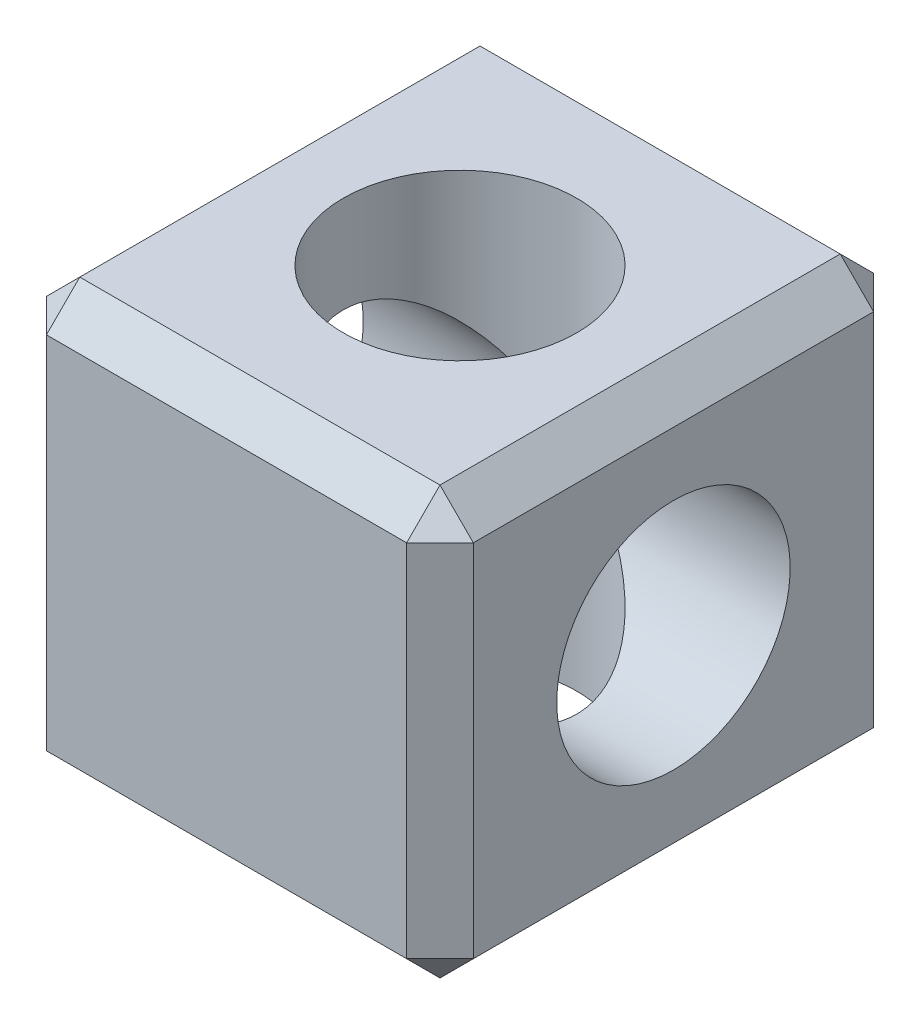
from build123d import *

# Parameters (mm, degrees)
BLOCK_PROFILE_SKETCH_W  = 64
BLOCK_PROFILE_SKETCH_H  = 64
BLOCK_BODY_DEPTH        = 70
CROSS_HOLE_A_SKETCH_R   = 17.5
CROSS_HOLE_A_DEPTH      = 101.09995005
CROSS_HOLE_B_SKETCH_R   = 17.5
CROSS_HOLE_B_DEPTH      = 101.09995005
EDGE_CHAMFERS_5X45_SIZE = 5


with BuildPart() as part:
    # Block Profile Sketch → Block Body (new body)
    with BuildSketch(Plane.XY):
        Rectangle(BLOCK_PROFILE_SKETCH_W, BLOCK_PROFILE_SKETCH_H)
    extrude(amount=BLOCK_BODY_DEPTH)

    # Cross Hole A Sketch → Cross Hole A (cut, through all)
    with BuildSketch(Plane(origin=(0, 32, 0), x_dir=(1, 0, 0), z_dir=(0, 1, 0))):
        with Locations(Location((0, -35, 0), (0, 0, 180))):
            Circle(CROSS_HOLE_A_SKETCH_R)
    extrude(amount=-CROSS_HOLE_A_DEPTH, mode=Mode.SUBTRACT)

    # Cross Hole B Sketch → Cross Hole B (cut, through all)
    with BuildSketch(Plane(origin=(32, 0, 0), x_dir=(0, 0, -1), z_dir=(1, 0, 0))):
        with Locations(Location((-35, 0, 0), (0, 0, 90))):
            Circle(CROSS_HOLE_B_SKETCH_R)
    extrude(amount=-CROSS_HOLE_B_DEPTH, mode=Mode.SUBTRACT)

    # Edge Chamfers 5x45°
    edge_chamfers_5x45_edges = [part.edges().sort_by_distance(p)[0] for p in [
        (32, 0, 70),
        (0, 32, 70),
        (-32, 0, 70),
        (0, 32, 0),
        (32, 0, 0),
        (-32, 0, 0),
        (-32, 32, 35),
        (32, 32, 35),
        (32, -32, 35),
        (-32, -32, 35),
        (0, -32, 70),
    ]]
    chamfer(edge_chamfers_5x45_edges, length=EDGE_CHAMFERS_5X45_SIZE)


solid = part.part
